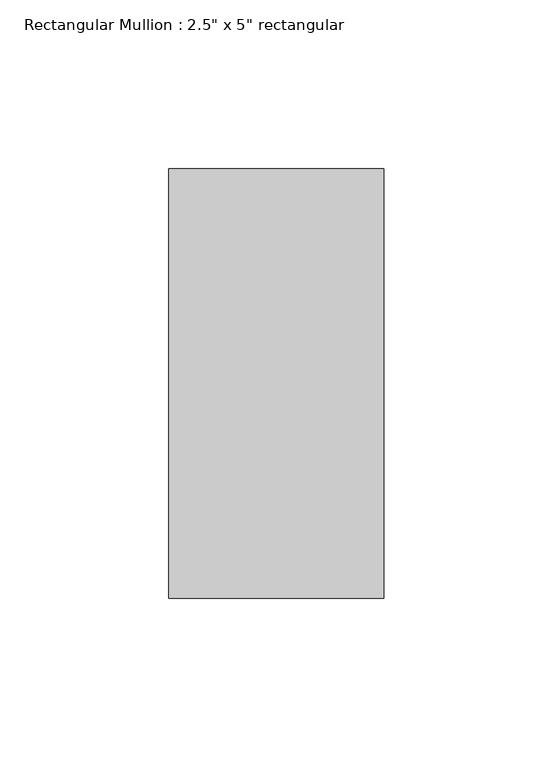
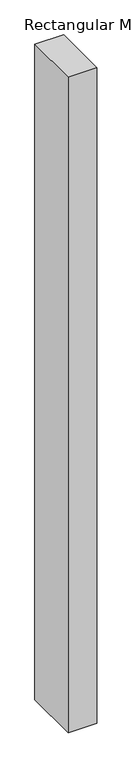
"""IFC4 building model written with IfcOpenShell, lengths in millimetres: member geometry."""

from ifc_helpers import new_model, si_unit, frame, origin, place, context, project, spatial, polyline, outline, extrude, source, transform, mapped, element, save


def member_032a0f9a(model_context):
    return source(origin(), model_context, "Body", "SweptSolid", [
        extrude(outline(polyline([(31.75, 63.5), (31.75, -63.5), (-31.75, -63.5), (-31.75, 63.5), (31.75, 63.5)])), frame((0.0, 0.0, -1529.8884341), z_axis=(0.0, 0.0, 1.0), x_axis=(1.0, 0.0, 0.0)), (0.0, 0.0, 1.0), 1529.8884341),
    ])


if __name__ == "__main__":
    model = new_model("IFC4")
    model_context = context("Model", 3, world=origin())
    ifc_project = project(units=[si_unit("LENGTHUNIT", "METRE", prefix="MILLI")], contexts=[model_context])
    site = spatial("IfcSite", under=ifc_project)
    building = spatial("IfcBuilding", under=site)
    placement = place(None, origin())
    member_shape = member_032a0f9a(model_context)
    element("IfcMember", 1, ObjectType="Rectangular Mullion : 2.5\" x 5\" rectangular", at=placement, inside=building, context=model_context, shape_type="MappedRepresentation", body=[
        mapped(member_shape, transform((0.0, 0.0, 0.0), x_axis=(1.0, 0.0, 0.0), y_axis=(0.0, 1.0, 0.0), z_axis=(0.0, 0.0, 1.0))),
    ])
    save(model, "model.ifc")

# Revit data of these elements
# Type "Rectangular Mullion : 2.5\" x 5\" rectangular"
#   built-in parameter 1007304 = 0.416667 (stored number, unit not read)
#   built-in parameter 1007301 = 0.104167 (stored number, unit not read)
#   built-in parameter 1007300 = 0.104167 (stored number, unit not read)
# Element 1 (IfcMember, "Rectangular Mullion : 2.5\" x 5\" rectangular")
#   Materials on its faces: "Aluminum"
# Materials
#   "Aluminum": class "Metal", colour RGB 247 247 247, transparency 0, Description = "Aluminum 6061", Cost = 0
